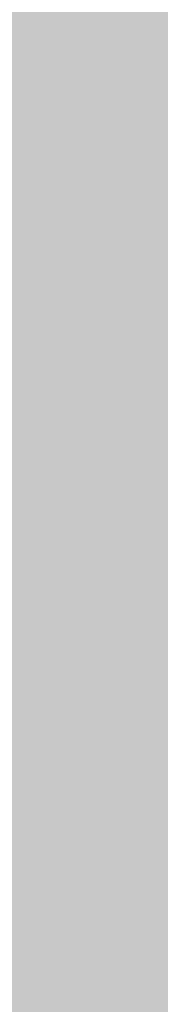
# Model space of a CAD drawing. Units: inches. Extents: x 2083 to 3317, y 1141 to 2115.
# Tile 179 of 256: x 3126.94671 to 3126.95594, y 1263.29018 to 1263.35483. Entities that reach past the tile are written whole.
import ezdxf

# ---------------------------------------------------------------- set-up
doc = ezdxf.new("R2010")
doc.units = ezdxf.units.IN
doc.layers.add('A-ANNO-DIMS', color=2, linetype='Continuous', lineweight=18)
doc.layers.add('A-WALL-PATT', color=251, linetype='Continuous', lineweight=13, true_color=0x636466)
doc.styles.get("Standard").update_dxf_attribs({"font": 'arial.ttf'})
doc.dimstyles.new('ISO-25', dxfattribs={"dimtxt": 12, "dimasz": 12, "dimexe": 1.25, "dimexo": 0.625, "dimtad": 1, "dimlunit": 3, "dimtxsty": 'Standard', "dimcen": 2.5, "dimadec": 0, "dimazin": 0, "dimtfac": 1, "dimtmove": 0, "dimatfit": 3, "dimfxl": 1, "dimarcsym": 0})

# ---------------------------------------------------------------- blocks, each defined once
blk = doc.blocks.new('*D26')
at = {"layer": 'A-ANNO-DIMS', "color": 0, "lineweight": -2, "transparency": 16777216}
for p, q in [((3088.985844, 1274.915092), (3088.985844, 1270.951963)), ((3111.240037, 1274.915092), (3111.240037, 1270.951963)), ((3076.985844, 1272.201963), (2840.262447, 1272.201963)), ((3111.240037, 1272.201963), (3088.985844, 1272.201963)), ((3123.240037, 1272.201963), (3135.240037, 1272.201963))]:
    blk.add_line(p, q, dxfattribs=at)
at = {"layer": 'A-ANNO-DIMS', "color": 0, "transparency": 16777216}
for points in [[(3076.985844, 1274.201963), (3076.985844, 1270.201963), (3088.985844, 1272.201963)], [(3123.240037, 1274.201963), (3123.240037, 1270.201963), (3111.240037, 1272.201963)]]:
    blk.add_solid(points, dxfattribs=at)
at = {"layer": 'Defpoints', "color": 0, "transparency": 16777216}
for p in [(3088.985844, 1275.540092), (3111.240037, 1275.540092), (3088.985844, 1272.201963)]:
    blk.add_point(p, dxfattribs=at)
at = {"layer": 'A-ANNO-DIMS', "color": 0, "transparency": 16777216, "insert": (2952.624146, 1279.031602), "char_height": 12, "attachment_point": 5}
blk.add_mtext('NIGHTSTAND 1\'-10 1/2" TYP.', dxfattribs=at)
blk = doc.blocks.new('*D27')
at = {"layer": 'A-ANNO-DIMS', "color": 0, "lineweight": -2, "transparency": 16777216}
for p, q in [((3114.578165, 1309.794285), (3114.578165, 1321.794285)), ((3111.865037, 1297.794285), (3115.828165, 1297.794285)), ((3114.578165, 1297.794285), (3114.578165, 1275.540092)), ((3111.865037, 1275.540092), (3115.828165, 1275.540092)), ((3114.578165, 1263.540092), (3114.578165, 1140.988591))]:
    blk.add_line(p, q, dxfattribs=at)
at = {"layer": 'A-ANNO-DIMS', "color": 0, "transparency": 16777216}
for points in [[(3112.578165, 1309.794285), (3116.578165, 1309.794285), (3114.578165, 1297.794285)], [(3112.578165, 1263.540092), (3116.578165, 1263.540092), (3114.578165, 1275.540092)]]:
    blk.add_solid(points, dxfattribs=at)
at = {"layer": 'Defpoints', "color": 0, "transparency": 16777216}
for p in [(3111.240037, 1297.794285), (3111.240037, 1275.540092), (3114.578165, 1275.540092)]:
    blk.add_point(p, dxfattribs=at)
at = {"layer": 'A-ANNO-DIMS', "color": 0, "transparency": 16777216, "insert": (3107.748527, 1196.264342), "char_height": 12, "attachment_point": 5, "rotation": 90}
blk.add_mtext('1\'-10 1/2" TYP.', dxfattribs=at)

msp = doc.modelspace()

# ---------------------------------------------------------------- hatches: boundary and pattern name
at = {"layer": 'A-WALL-PATT'}
h = msp.add_hatch(color=256, dxfattribs=at)
h.dxf.hatch_style = 1
h.paths.add_polyline_path([(3126.959783, 2020.76136), (2748.959783, 2020.76136), (2604.959783, 2020.76136), (2226.959783, 2020.76136), (2226.959783, 1702.76136), (2466.959783, 1702.76136), (2466.959783, 1582.76136), (2418.959783, 1582.76136), (2418.959783, 1477.76136), (2226.959783, 1477.76136), (2226.959783, 1263.26136), (2544.959783, 1263.26136), (2544.959783, 1411.76136), (2604.959783, 1411.76136), (2685.959783, 1411.76136), (2685.959783, 1420.76136), (2604.959783, 1420.76136), (2604.959783, 1573.76136), (2604.959783, 1702.76136), (2604.959783, 2011.76136), (2748.959783, 2011.76136), (2748.959783, 1702.76136), (2862.959783, 1702.76136), (2862.959783, 1621.76136), (2871.959783, 1621.76136), (2871.959783, 1702.76136), (2883.959783, 1702.76136), (2883.959783, 1706.939459, -0.026459), (2883.959783, 1711.76136), (2757.959783, 1711.76136), (2757.959783, 1807.76136), (2787.959783, 1807.76136), (2787.959783, 1812.26136), (2757.959783, 1812.26136), (2757.959783, 2011.76136), (2877.959783, 2011.76136), (2877.959783, 1812.26136), (2847.959783, 1812.26136), (2847.959783, 1807.76136), (2889.835742, 1807.76136), (2889.835742, 1812.26136), (2882.459783, 1812.26136), (2882.459783, 2011.76136), (3117.959783, 2011.76136), (3117.959783, 1812.26136), (2937.835742, 1812.26136), (2937.835742, 1807.76136), (2995.709783, 1807.76136), (2995.709783, 1796.117666), (3000.209783, 1796.117666), (3000.209783, 1807.76136), (3117.959783, 1807.76136), (3117.959783, 1711.76136), (3000.209783, 1711.76136), (3000.209783, 1760.117666), (2998.572705, 1760.117666, -0.020711), (2995.709783, 1760.117666), (2995.709783, 1711.76136), (2931.959783, 1711.76136), (2931.959783, 1702.76136), (3126.959783, 1702.76136)])
h.paths.add_polyline_path([(2471.459783, 2011.76136), (2471.459783, 1810.01136), (2462.716936, 1810.01136), (2462.716936, 1805.51136), (2505.959783, 1805.51136), (2505.959783, 1810.01136), (2475.959783, 1810.01136), (2475.959783, 2011.76136), (2595.959783, 2011.76136), (2595.959783, 1810.01136), (2565.959783, 1810.01136), (2565.959783, 1805.51136), (2595.959783, 1805.51136), (2595.959783, 1711.76136), (2235.959783, 1711.76136), (2235.959783, 1805.51136), (2353.709783, 1805.51136), (2353.709783, 1796.054162), (2358.209783, 1796.054162), (2358.209783, 1805.51136), (2414.716936, 1805.51136), (2414.716936, 1810.01136), (2235.959783, 1810.01136), (2235.959783, 2011.76136)], flags=16)
h.paths.add_polyline_path([(2270.204734, 1994.610008), (2270.204734, 1970.610008), (2246.204734, 1970.610008), (2246.204734, 1994.610008)], flags=0)
edge = h.paths.add_edge_path(flags=0)
edge.add_ellipse((2332.027391, 1899.798176), major_axis=(-3.042994, 3.042994), ratio=0.16825245, start_angle=-161.332166, end_angle=-156.307114, ccw=False)
edge.add_ellipse((2333.082037, 1898.74353), major_axis=(-1.054646, 1.054646), ratio=0.4535321, start_angle=-123.371019, end_angle=-94.159107)
edge = h.paths.add_edge_path(flags=0)
edge.add_ellipse((2332.027391, 1968.87629), major_axis=(3.042994, 3.042994), ratio=0.16825245, start_angle=18.667834, end_angle=23.692886)
edge.add_spline(control_points=[(2332.925596, 1970.691105), (2332.226768, 1970.3361), (2330.893709, 1969.658905), (2328.41308, 1970.932138), (2327.203934, 1967.748712), (2324.709596, 1969.955589), (2322.532822, 1967.012354), (2320.012846, 1971.295812), (2317.680308, 1968.157845), (2316.040526, 1967.102047), (2315.426904, 1966.809602)], knot_values=[0, 0, 0, 0, 2.267059, 4.324559, 6.685584, 8.878641, 11.121502, 14.300359, 17.755284, 19.732645, 19.732645, 19.732645, 19.732645], degree=3, periodic=0)
edge.add_ellipse((2332.027391, 1968.87629), major_axis=(3.042994, 3.042994), ratio=0.16825245, start_angle=18.667834, end_angle=23.692886, ccw=False)
edge.add_ellipse((2333.082037, 1969.930936), major_axis=(1.054646, 1.054646), ratio=0.4535321, start_angle=56.628981, end_angle=85.840893, ccw=False)
edge = h.paths.add_edge_path(flags=0)
edge.add_spline(control_points=[(2296.428287, 1967.987908), (2293.627804, 1965.336314), (2287.703624, 1959.727094), (2299.74386, 1949.995699), (2294.532591, 1935.668528), (2290.573228, 1920.603512), (2293.394124, 1909.973691), (2296.185407, 1904.966543)], knot_values=[0.099185, 0.099185, 0.099185, 0.099185, 0.345301, 0.619822, 0.982653, 1.386093, 1.810555, 1.810555, 1.810555, 1.810555], degree=3, periodic=0)
edge.add_spline(control_points=[(2296.185407, 1904.966543), (2297.383582, 1902.6193), (2298.000969, 1901.949312), (2298.55297, 1901.468155)], knot_values=[0.006246, 0.006246, 0.006246, 0.006246, 0.055476, 0.055476, 0.055476, 0.055476], degree=3, periodic=0)
edge.add_spline(control_points=[(2298.55297, 1901.468155), (2297.258612, 1900.923224), (2295.225294, 1900.232126), (2293.060229, 1900.614205), (2292.101423, 1900.788415), (2292.089578, 1900.790568)], knot_values=[0.312835, 0.312835, 0.312835, 0.312835, 0.40178, 0.474987, 0.475903, 0.475903, 0.475903, 0.475903], degree=3, periodic=0)
edge.add_arc((2292.793646, 1904.664109), 3.937008, 215.420897, 259.698179, ccw=False)
edge.add_spline(control_points=[(2289.585314, 1902.382304), (2289.476652, 1902.535087), (2289.36848, 1902.688035), (2289.260865, 1902.84117)], knot_values=[0.102872, 0.102872, 0.102872, 0.102872, 0.116896, 0.116896, 0.116896, 0.116896], degree=3, periodic=0)
edge.add_spline(control_points=[(2289.260865, 1902.84117), (2288.686604, 1902.550192), (2287.640048, 1902.019902), (2285.881337, 1901.873954), (2283.852972, 1901.504352), (2281.719987, 1899.710538), (2278.466991, 1899.492942), (2276.157136, 1901.883202), (2272.258953, 1899.804071), (2267.777605, 1901.843183), (2262.243882, 1900.184033), (2257.414927, 1901.782061), (2254.318374, 1900.72612), (2253.178285, 1900.337343)], knot_values=[0, 0, 0, 0, 1.907977, 3.477176, 5.261074, 7.972851, 11.680248, 13.717921, 16.939592, 22.789562, 27.502503, 33.595215, 37.145618, 37.145618, 37.145618, 37.145618], degree=3, periodic=0)
edge.add_line((2253.178285, 1900.337343), (2250.24424, 1902.84117))
edge.add_line((2250.24424, 1902.84117), (2250.24424, 1965.833296))
edge.add_line((2250.24424, 1965.833296), (2253.178285, 1968.337123))
edge.add_spline(control_points=[(2253.178285, 1968.337123), (2254.318374, 1967.948346), (2257.414927, 1966.892405), (2262.243882, 1968.490433), (2267.777605, 1966.831283), (2271.52673, 1968.537217), (2273.875914, 1967.828289), (2274.206701, 1967.727642)], knot_values=[0, 0, 0, 0, 0.09018, 0.244935, 0.364644, 0.513233, 0.537855, 0.537855, 0.537855, 0.537855], degree=3, periodic=0)
edge.add_arc((2274.352887, 1963.793349), 3.937008, 72.051134, 92.127949, ccw=False)
edge.add_arc((2281.296933, 1985.230003), 18.596298, 252.0511336, 288.5657217)
edge.add_arc((2292.316717, 1956.02888), 12.646081, 71.0267879, 113.7782184, ccw=False)
edge = h.paths.add_edge_path(flags=0)
edge.add_spline(control_points=[(2274.899415, 1951.856195), (2275.066156, 1951.616592), (2275.232687, 1951.376588), (2275.397987, 1951.135855)], knot_values=[1.409916, 1.409916, 1.409916, 1.409916, 1.43159, 1.43159, 1.43159, 1.43159], degree=3, periodic=0)
edge.add_spline(control_points=[(2275.397987, 1951.135855), (2275.792106, 1950.561885), (2276.179231, 1949.983774), (2276.545546, 1949.397103)], knot_values=[1.358238, 1.358238, 1.358238, 1.358238, 1.409916, 1.409916, 1.409916, 1.409916], degree=3, periodic=0)
edge.add_line((2276.545546, 1949.397103), (2277.437289, 1947.862185))
edge.add_spline(control_points=[(2277.437289, 1947.862185), (2276.303834, 1945.673115), (2274.639698, 1942.426882), (2274.631615, 1938.0939), (2272.799124, 1930.85155), (2274.356426, 1943.897046), (2275.947681, 1947.923356), (2276.545546, 1949.397103)], knot_values=[0.005632, 0.005632, 0.005632, 0.005632, 0.186014, 0.266002, 0.357087, 0.59639, 0.739732, 0.739732, 0.739732, 0.739732], degree=3, periodic=0)
edge.add_spline(control_points=[(2276.545546, 1949.397103), (2276.179231, 1949.983774), (2275.792106, 1950.561885), (2275.397987, 1951.135855)], knot_values=[1.358238, 1.358238, 1.358238, 1.358238, 1.409916, 1.409916, 1.409916, 1.409916], degree=3, periodic=0)
edge.add_spline(control_points=[(2275.397987, 1951.135855), (2274.9425, 1950.080452), (2274.20776, 1948.025272), (2273.934602, 1944.851477), (2272.468534, 1937.627489), (2273.466216, 1945.696466), (2274.700615, 1951.059472), (2274.899415, 1951.856195)], knot_values=[0.104364, 0.104364, 0.104364, 0.104364, 0.189636, 0.269624, 0.36071, 0.600013, 0.644622, 0.644622, 0.644622, 0.644622], degree=3, periodic=0)
h.paths.add_polyline_path([(2269.167514, 1963.127573, -0.357527), (2268.170633, 1960.97637, -0.092561), (2268.170633, 1939.436325, -0.357527), (2269.167514, 1937.285122, -0.357527), (2267.01631, 1938.282002, -0.164785), (2254.685581, 1938.282002, -0.357527), (2252.534378, 1937.285122, -0.357527), (2253.531259, 1939.436325, -0.092561), (2253.531259, 1960.97637, -0.357527), (2252.534378, 1963.127573, -0.357527), (2254.685581, 1962.130692, -0.164785), (2267.01631, 1962.130692, -0.357527)], flags=0)
h.paths.add_polyline_path([(2248.874068, 1967.8018), (2248.874068, 1957.02771), (2249.457783, 1957.02771), (2249.457783, 1911.646756), (2248.874068, 1911.646756), (2248.874068, 1900.872666), (2246.511863, 1900.872666, 0.197327), (2244.149658, 1902.456873), (2244.149658, 1966.217592, 0.197327), (2246.511863, 1967.8018)], flags=0)
h.paths.add_polyline_path([(2269.167514, 1931.389344, -0.357527), (2268.170633, 1929.238141, -0.092561), (2268.170633, 1907.698096, -0.357527), (2269.167514, 1905.546893, -0.357527), (2267.01631, 1906.543774, -0.164785), (2254.685581, 1906.543774, -0.357527), (2252.534378, 1905.546893, -0.357527), (2253.531259, 1907.698096, -0.092561), (2253.531259, 1929.238141, -0.357527), (2252.534378, 1931.389344, -0.357527), (2254.685581, 1930.392463, -0.164785), (2267.01631, 1930.392463, -0.357527)], flags=0)
edge = h.paths.add_edge_path(flags=0)
edge.add_spline(control_points=[(2276.196858, 1906.723702), (2276.168144, 1909.028928), (2276.114049, 1913.371852), (2270.598417, 1924.924978), (2273.905175, 1919.012779), (2275.921711, 1916.262063), (2275.47457, 1912.402149), (2277.257874, 1910.380621), (2276.696044, 1908.225036), (2276.646218, 1906.813023), (2276.617825, 1906.008407)], knot_values=[0, 0, 0, 0, 8.61026, 16.221274, 18.843057, 23.804898, 27.440828, 29.356102, 31.203478, 33.650687, 33.650687, 33.650687, 33.650687], degree=3, periodic=0)
edge.add_spline(control_points=[(2276.617825, 1906.008407), (2276.623313, 1905.624144), (2276.497738, 1904.628661), (2275.441779, 1903.854725), (2274.937314, 1903.08045), (2274.85908, 1902.84117)], knot_values=[0.156488, 0.156488, 0.156488, 0.156488, 0.184398, 0.231376, 0.250598, 0.250598, 0.250598, 0.250598], degree=3, periodic=0)
edge.add_line((2274.85908, 1902.84117), (2276.50598, 1902.84117))
edge.add_spline(control_points=[(2276.50598, 1902.84117), (2276.788308, 1903.08494), (2277.665071, 1904.125196), (2278.249538, 1904.340738), (2277.653872, 1908.527387), (2278.15567, 1906.227808), (2278.100464, 1905.285948), (2278.846675, 1904.069005), (2277.856785, 1903.414948), (2277.874191, 1902.99105), (2277.903562, 1902.84117)], knot_values=[0.059574, 0.059574, 0.059574, 0.059574, 0.080753, 0.103741, 0.16972, 0.176036, 0.207137, 0.240474, 0.262341, 0.27366, 0.27366, 0.27366, 0.27366], degree=3, periodic=0)
edge.add_line((2277.903562, 1902.84117), (2280.029825, 1902.84117))
edge.add_spline(control_points=[(2280.029825, 1902.84117), (2279.888221, 1903.088398), (2279.499257, 1903.981551), (2280.152284, 1905.939349), (2278.103615, 1909.657757), (2279.762395, 1907.185285), (2280.3279, 1904.874861), (2280.485109, 1903.48959), (2281.463269, 1903.249432), (2281.758343, 1902.936497), (2281.834036, 1902.84117)], knot_values=[0.013856, 0.013856, 0.013856, 0.013856, 0.034874, 0.088867, 0.107879, 0.126738, 0.158714, 0.193757, 0.217487, 0.226722, 0.226722, 0.226722, 0.226722], degree=3, periodic=0)
edge.add_spline(control_points=[(2281.834036, 1902.84117), (2281.787535, 1902.826703), (2281.647022, 1902.782988), (2281.395527, 1902.85949), (2281.088077, 1902.985242), (2280.720683, 1903.060902), (2280.333451, 1903.025726), (2280.124767, 1902.898879), (2280.029825, 1902.84117)], knot_values=[0, 0, 0, 0, 0.14413, 0.435517, 0.749276, 1.153046, 1.548371, 1.878348, 1.878348, 1.878348, 1.878348], degree=3, periodic=0)
edge.add_line((2280.029825, 1902.84117), (2277.903562, 1902.84117))
edge.add_spline(control_points=[(2277.903562, 1902.84117), (2277.892855, 1902.795855), (2277.865396, 1902.679637), (2277.607479, 1902.687483), (2277.27405, 1902.8007), (2276.837921, 1902.619775), (2276.583807, 1902.789261), (2276.50598, 1902.84117)], knot_values=[0, 0, 0, 0, 0.127189, 0.326199, 0.628009, 1.24357, 1.515331, 1.515331, 1.515331, 1.515331], degree=3, periodic=0)
edge.add_line((2276.50598, 1902.84117), (2274.85908, 1902.84117))
edge.add_spline(control_points=[(2274.85908, 1902.84117), (2274.814437, 1902.898587), (2274.72513, 1903.013446), (2274.493477, 1903.118968), (2274.244285, 1902.960539), (2273.937121, 1903.184942), (2273.614039, 1902.983143), (2273.408316, 1902.883045), (2273.322254, 1902.84117)], knot_values=[0, 0, 0, 0, 0.21843, 0.436957, 0.687977, 0.990379, 1.398396, 1.69185, 1.69185, 1.69185, 1.69185], degree=3, periodic=0)
edge.add_spline(control_points=[(2273.322254, 1902.84117), (2273.61674, 1903.445692), (2274.273998, 1904.538253), (2276.027239, 1904.573702), (2276.206963, 1906.583637), (2276.196858, 1906.723702)], knot_values=[0.012227, 0.012227, 0.012227, 0.012227, 0.059472, 0.106218, 0.134458, 0.134458, 0.134458, 0.134458], degree=3, periodic=0)
h.paths.add_polyline_path([(2270.776054, 1897.789828), (2270.776054, 1873.789828), (2246.776054, 1873.789828), (2246.776054, 1897.789828)], flags=0)
h.paths.add_polyline_path([(2353.709783, 1760.005059), (2353.709783, 1760.054162), (2358.209783, 1760.054162, -0.033729)], flags=0)
h.paths.add_polyline_path([(2321.819119, 1737.529186), (2341.995327, 1737.529186, -0.414214), (2343.203273, 1736.321241), (2343.203273, 1721.020596, -0.414214), (2341.995327, 1719.812651), (2321.819119, 1719.812651, -0.414214), (2320.611173, 1721.020596), (2320.611173, 1736.321241, -0.414214)], flags=0)
h.paths.add_polyline_path([(2324.23501, 1736.321241), (2339.579436, 1736.321241, -0.414214), (2341.995327, 1733.905349), (2341.995327, 1725.44973, -0.414214), (2339.579436, 1723.033839), (2333.680588, 1723.033839), (2333.845317, 1722.045467, -0.870646), (2335.425399, 1721.825893, -0.767327), (2333.922694, 1721.423245), (2331.291024, 1721.423245, -0.767327), (2329.788319, 1721.825893, -0.870646), (2331.368401, 1722.045467), (2331.53313, 1723.033839), (2324.23501, 1723.033839, -0.414214), (2321.819119, 1725.44973), (2321.819119, 1733.905349, -0.414214)], flags=0)
h.paths.add_polyline_path([(2570.483789, 1928.615444), (2589.683789, 1928.615444), (2590.168829, 1928.615444), (2590.168829, 1904.993397), (2570.483789, 1904.993397)], flags=0)
h.paths.add_polyline_path([(2574.447324, 1927.263822, -1), (2572.828836, 1927.263822, -1)], flags=0)
h.paths.add_polyline_path([(2573.089867, 1926.940877), (2573.925032, 1927.776042), (2574.147743, 1927.553332), (2573.312577, 1926.718166)], flags=0)
h.paths.add_polyline_path([(2578.779065, 1919.729618, -1), (2571.591663, 1919.729618, -1)], flags=0)
h.paths.add_polyline_path([(2578.385364, 1919.729618, -1), (2571.985364, 1919.729618, -1)], flags=0)
h.paths.add_polyline_path([(2331.595764, 1729.476216, -1), (2333.617954, 1729.476216, -1)], flags=0)
h.paths.add_polyline_path([(2578.034228, 1927.263822, -1), (2576.41574, 1927.263822, -1)], flags=0)
h.paths.add_polyline_path([(2576.688851, 1927.531089), (2576.911562, 1927.753799), (2577.746728, 1926.918634), (2577.524017, 1926.695923)], flags=0)
h.paths.add_polyline_path([(2578.139065, 1909.859539, -1), (2572.231663, 1909.859539, -1)], flags=0)
h.paths.add_polyline_path([(2577.745364, 1909.859539, -1), (2572.625364, 1909.859539, -1)], flags=0)
h.paths.add_polyline_path([(2583.797718, 1927.263822, -1), (2582.179229, 1927.263822, -1)], flags=0)
h.paths.add_polyline_path([(2582.718649, 1927.753799), (2583.553814, 1926.918634), (2583.331103, 1926.695923), (2582.495938, 1927.531089)], flags=0)
h.paths.add_polyline_path([(2582.495938, 1927.531089), (2582.718649, 1927.753799), (2583.553814, 1926.918634), (2583.331103, 1926.695923)], flags=0)
h.paths.add_polyline_path([(2587.739065, 1920.529618, -1), (2581.831663, 1920.529618, -1)], flags=0)
h.paths.add_polyline_path([(2587.345364, 1920.529618, -1), (2582.225364, 1920.529618, -1)], flags=0)
h.paths.add_polyline_path([(2587.384622, 1927.263822, -1), (2585.766133, 1927.263822, -1)], flags=0)
h.paths.add_polyline_path([(2586.081993, 1926.980247), (2586.917158, 1927.815412), (2587.139869, 1927.592702), (2586.304703, 1926.757536)], flags=0)
h.paths.add_polyline_path([(2588.379065, 1910.659539, -1), (2581.191663, 1910.659539, -1)], flags=0)
h.paths.add_polyline_path([(2587.985364, 1910.659539, -1), (2581.585364, 1910.659539, -1)], flags=0)
h.paths.add_polyline_path([(2417.167729, 1729.477895), (2437.343937, 1729.477895, -0.414214), (2438.551883, 1728.26995), (2438.551883, 1712.969306, -0.414214), (2437.343937, 1711.76136), (2417.167729, 1711.76136, -0.414214), (2415.959783, 1712.969306), (2415.959783, 1728.26995, -0.414214)], flags=0)
h.paths.add_polyline_path([(2419.58362, 1728.26995), (2434.928046, 1728.26995, -0.414214), (2437.343937, 1725.854059), (2437.343937, 1717.39844, -0.414214), (2434.928046, 1714.982548), (2429.029199, 1714.982548), (2429.193927, 1713.994176, -0.870646), (2430.774009, 1713.774603, -0.767327), (2429.271304, 1713.371954), (2426.639634, 1713.371954, -0.767327), (2425.136929, 1713.774603, -0.870646), (2426.717011, 1713.994176), (2426.88174, 1714.982548), (2419.58362, 1714.982548, -0.414214), (2417.167729, 1717.39844), (2417.167729, 1725.854059, -0.414214)], flags=0)
h.paths.add_polyline_path([(2419.58362, 1728.26995), (2434.928046, 1728.26995, -0.414214), (2437.343937, 1725.854059), (2437.343937, 1717.39844, -0.414214), (2434.928046, 1714.982548), (2429.029199, 1714.982548), (2428.358118, 1719.009034), (2427.552821, 1719.009034), (2426.88174, 1714.982548), (2419.58362, 1714.982548, -0.414214), (2417.167729, 1717.39844), (2417.167729, 1725.854059, -0.414214)], flags=0)
h.paths.add_polyline_path([(2426.944374, 1721.424925, -1), (2428.966564, 1721.424925, -1)], flags=0)
h.paths.add_polyline_path([(2475.959783, 1702.76136), (2595.959783, 1702.76136), (2595.959783, 1582.76136), (2475.959783, 1582.76136)], flags=16)
h.paths.add_polyline_path([(2427.959783, 1573.76136), (2595.959783, 1573.76136), (2595.959783, 1468.76136), (2595.959783, 1420.76136), (2384.459783, 1420.76136), (2384.459783, 1468.76136), (2427.959783, 1468.76136)], flags=16)
h.paths.add_polyline_path([(2379.959783, 1468.76136), (2379.959783, 1420.76136), (2235.959783, 1420.76136), (2235.959783, 1468.76136)], flags=16)
h.paths.add_polyline_path([(2317.815996, 1466.695767), (2337.992205, 1466.695767, -0.414214), (2339.20015, 1465.487821), (2339.20015, 1450.187177, -0.414214), (2337.992205, 1448.979232), (2317.815996, 1448.979232, -0.414214), (2316.608051, 1450.187177), (2316.608051, 1465.487821, -0.414214)], flags=0)
h.paths.add_polyline_path([(2320.231887, 1465.487821), (2335.576313, 1465.487821, -0.414214), (2337.992205, 1463.07193), (2337.992205, 1454.616311, -0.414214), (2335.576313, 1452.20042), (2329.677466, 1452.20042), (2329.842195, 1451.212047, -0.870646), (2331.422276, 1450.992474, -0.767327), (2329.919571, 1450.589826), (2327.287902, 1450.589826, -0.767327), (2325.785197, 1450.992474, -0.870646), (2327.365278, 1451.212047), (2327.530007, 1452.20042), (2320.231887, 1452.20042, -0.414214), (2317.815996, 1454.616311), (2317.815996, 1463.07193, -0.414214)], flags=0)
h.paths.add_polyline_path([(2320.231887, 1465.487821), (2335.576313, 1465.487821, -0.414214), (2337.992205, 1463.07193), (2337.992205, 1454.616311, -0.414214), (2335.576313, 1452.20042), (2329.677466, 1452.20042), (2329.006385, 1456.226905), (2328.201088, 1456.226905), (2327.530007, 1452.20042), (2320.231887, 1452.20042, -0.414214), (2317.815996, 1454.616311), (2317.815996, 1463.07193, -0.414214)], flags=0)
h.paths.add_polyline_path([(2327.592641, 1458.642796, -1), (2329.614832, 1458.642796, -1)], flags=0)
h.paths.add_polyline_path([(2244.411744, 1433.340453), (2241.920945, 1433.340453, -0.414214), (2240.017856, 1435.243542), (2240.017856, 1440.952808, -0.414211), (2241.920925, 1442.855897), (2244.411744, 1442.855897, -1.976472)], flags=0)
h.paths.add_polyline_path([(2245.356888, 1434.397536, -0.414214), (2245.356888, 1441.798814, -2.144098)], flags=0)
h.paths.add_polyline_path([(2535.959783, 1416.26136), (2535.959783, 1272.26136), (2235.959783, 1272.26136), (2235.959783, 1416.26136)], flags=16)
h.paths.add_polyline_path([(2260.119561, 1384.292841), (2260.119561, 1362.038649), (2237.865369, 1362.038649), (2237.865369, 1384.292841)], flags=0)
edge = h.paths.add_edge_path(flags=0)
edge.add_line((2318.251847, 1362.093298), (2318.145797, 1362.000973))
edge.add_ellipse((2317.445116, 1360.431044), major_axis=(2.82164, 2.82164), ratio=0.16825245, start_angle=18.667834, end_angle=20.948127, ccw=False)
edge.add_ellipse((2318.423045, 1361.408974), major_axis=(0.977929, 0.977929), ratio=0.4535321, start_angle=56.628981, end_angle=70.226201, ccw=False)
edge = h.paths.add_edge_path(flags=0)
edge.add_line((2319.10737, 1295.571078), (2319.015044, 1295.677128))
edge.add_ellipse((2317.445116, 1296.377809), major_axis=(-2.82164, 2.82164), ratio=0.16825245, start_angle=-161.332166, end_angle=-159.051873, ccw=False)
edge.add_ellipse((2318.423045, 1295.39988), major_axis=(-0.977929, 0.977929), ratio=0.4535321, start_angle=-123.371019, end_angle=-109.773799)
edge = h.paths.add_edge_path(flags=0)
edge.add_spline(control_points=[(2284.210349, 1301.170219), (2284.580688, 1300.444719), (2284.891189, 1299.892024), (2285.159553, 1299.461018)], knot_values=[0.039066, 0.039066, 0.039066, 0.039066, 0.055476, 0.055476, 0.055476, 0.055476], degree=3, periodic=0)
edge.add_line((2285.159553, 1299.461018), (2284.210349, 1301.170219))
edge = h.paths.add_edge_path(flags=0)
edge.add_line((2280.412458, 1297.298013), (2283.369991, 1297.036122))
edge.add_line((2283.369991, 1297.036122), (2286.40569, 1297.92631))
edge.add_spline(control_points=[(2286.40569, 1297.92631), (2285.305487, 1297.463119), (2284.344777, 1297.129151), (2283.369991, 1297.036122)], knot_values=[0.394369, 0.394369, 0.394369, 0.394369, 0.475903, 0.475903, 0.475903, 0.475903], degree=3, periodic=0)
edge.add_spline(control_points=[(2283.369991, 1297.036122), (2283.28139, 1297.027666), (2282.316289, 1296.957336), (2281.312502, 1297.134479), (2280.423441, 1297.296016), (2280.412458, 1297.298013)], knot_values=[0.312835, 0.312835, 0.312835, 0.312835, 0.320246, 0.393453, 0.394369, 0.394369, 0.394369, 0.394369], degree=3, periodic=0)
edge = h.paths.add_edge_path(flags=0)
edge.add_line((2284.435561, 1359.607285), (2280.446291, 1355.328047))
edge.add_line((2280.446291, 1355.328047), (2279.579987, 1351.017754))
edge.add_line((2279.579987, 1351.017754), (2282.412974, 1346.580433))
edge.add_spline(control_points=[(2282.412974, 1346.580433), (2283.153331, 1345.589236), (2284.252896, 1344.028897), (2284.801037, 1342.387167), (2284.935162, 1341.805544)], knot_values=[1.240098, 1.240098, 1.240098, 1.240098, 1.332892, 1.382712, 1.382712, 1.382712, 1.382712], degree=3, periodic=0)
edge.add_spline(control_points=[(2284.935162, 1341.805544), (2285.319108, 1340.1406), (2285.233029, 1338.409204), (2284.909938, 1336.654122)], knot_values=[1.097484, 1.097484, 1.097484, 1.097484, 1.240098, 1.240098, 1.240098, 1.240098], degree=3, periodic=0)
edge.add_spline(control_points=[(2284.909938, 1336.654122), (2284.586848, 1334.89904), (2284.026745, 1333.120272), (2283.462644, 1331.360585)], knot_values=[0.95487, 0.95487, 0.95487, 0.95487, 1.097484, 1.097484, 1.097484, 1.097484], degree=3, periodic=0)
edge.add_line((2283.462644, 1331.360585), (2281.890376, 1326.153357))
edge.add_line((2281.890376, 1326.153357), (2280.756259, 1321.056089))
edge.add_line((2280.756259, 1321.056089), (2280.299205, 1316.001977))
edge.add_line((2280.299205, 1316.001977), (2280.715933, 1310.950068))
edge.add_line((2280.715933, 1310.950068), (2282.028094, 1305.972137))
edge.add_line((2282.028094, 1305.972137), (2284.210349, 1301.170219))
edge.add_spline(control_points=[(2284.210349, 1301.170219), (2283.340731, 1302.730185), (2282.611904, 1304.336493), (2282.028094, 1305.972137)], knot_values=[0.099185, 0.099185, 0.099185, 0.099185, 0.241799, 0.241799, 0.241799, 0.241799], degree=3, periodic=0)
edge.add_spline(control_points=[(2282.028094, 1305.972137), (2281.444283, 1307.60778), (2281.005489, 1309.272759), (2280.715933, 1310.950068)], knot_values=[0.241799, 0.241799, 0.241799, 0.241799, 0.384413, 0.384413, 0.384413, 0.384413], degree=3, periodic=0)
edge.add_spline(control_points=[(2280.715933, 1310.950068), (2280.433241, 1312.587613), (2280.289386, 1314.276959), (2280.298894, 1315.962032), (2280.299205, 1316.001977)], knot_values=[0.384413, 0.384413, 0.384413, 0.384413, 0.523647, 0.527028, 0.527028, 0.527028, 0.527028], degree=3, periodic=0)
edge.add_spline(control_points=[(2280.299205, 1316.001977), (2280.312326, 1317.686955), (2280.477871, 1319.367926), (2280.756259, 1321.056089)], knot_values=[0.527028, 0.527028, 0.527028, 0.527028, 0.669642, 0.669642, 0.669642, 0.669642], degree=3, periodic=0)
edge.add_spline(control_points=[(2280.756259, 1321.056089), (2281.034648, 1322.744252), (2281.42588, 1324.439608), (2281.890376, 1326.153357)], knot_values=[0.669642, 0.669642, 0.669642, 0.669642, 0.812256, 0.812256, 0.812256, 0.812256], degree=3, periodic=0)
edge.add_spline(control_points=[(2281.890376, 1326.153357), (2282.264383, 1327.533251), (2282.78787, 1329.26181), (2283.352751, 1331.01778), (2283.462644, 1331.360585)], knot_values=[0.812256, 0.812256, 0.812256, 0.812256, 0.927087, 0.95487, 0.95487, 0.95487, 0.95487], degree=3, periodic=0)
edge.add_line((2283.462644, 1331.360585), (2284.909938, 1336.654122))
edge.add_line((2284.909938, 1336.654122), (2284.935162, 1341.805544))
edge.add_line((2284.935162, 1341.805544), (2282.412974, 1346.580433))
edge.add_spline(control_points=[(2282.412974, 1346.580433), (2281.275127, 1348.103792), (2280.078447, 1349.570318), (2279.579987, 1351.017754)], knot_values=[1.382712, 1.382712, 1.382712, 1.382712, 1.525326, 1.525326, 1.525326, 1.525326], degree=3, periodic=0)
edge.add_spline(control_points=[(2279.579987, 1351.017754), (2279.443282, 1351.414721), (2279.136312, 1352.856922), (2279.73519, 1354.290385), (2280.446291, 1355.328047)], knot_values=[1.525326, 1.525326, 1.525326, 1.525326, 1.564439, 1.667941, 1.667941, 1.667941, 1.667941], degree=3, periodic=0)
edge.add_spline(control_points=[(2280.446291, 1355.328047), (2281.426113, 1356.757835), (2282.930837, 1358.18256), (2284.435561, 1359.607285)], knot_values=[1.667941, 1.667941, 1.667941, 1.667941, 1.810555, 1.810555, 1.810555, 1.810555], degree=3, periodic=0)
edge.add_arc((2280.623075, 1348.518181), 11.72618, 71.0267879, 113.7782184)
edge.add_arc((2270.404892, 1375.595156), 17.243567, 252.0511336, 288.5657217, ccw=False)
edge.add_arc((2263.965969, 1355.717847), 3.650622, 72.051134, 92.127949)
edge.add_arc((2263.965969, 1355.717847), 3.650622, 92.127949, 177.98513)
edge.add_spline(control_points=[(2260.317604, 1355.846199), (2260.260417, 1354.220668), (2260.551278, 1350.186547), (2262.999344, 1346.766251), (2264.472741, 1344.649024)], knot_values=[1.43159, 1.43159, 1.43159, 1.43159, 1.564144, 1.770695, 1.770695, 1.770695, 1.770695], degree=3, periodic=0)
edge.add_line((2264.472741, 1344.649024), (2264.93559, 1343.98253))
edge.add_spline(control_points=[(2263.801044, 1340.248105), (2263.843238, 1340.514088), (2264.067244, 1341.756465), (2264.512693, 1343.002453), (2264.935047, 1343.981083)], knot_values=[0.53657, 0.53657, 0.53657, 0.53657, 0.559349, 0.644622, 0.644622, 0.644622, 0.644622], degree=3, periodic=0)
edge.add_spline(control_points=[(2264.935047, 1343.981083), (2265.117771, 1343.714975), (2265.298875, 1343.447906), (2265.476756, 1343.179365)], knot_values=[1.384077, 1.384077, 1.384077, 1.384077, 1.409916, 1.409916, 1.409916, 1.409916], degree=3, periodic=0)
edge.add_spline(control_points=[(2265.476756, 1343.179365), (2265.654637, 1342.910823), (2265.829296, 1342.64081), (2265.99913, 1342.368812)], knot_values=[1.358238, 1.358238, 1.358238, 1.358238, 1.384077, 1.384077, 1.384077, 1.384077], degree=3, periodic=0)
edge.add_line((2265.99913, 1342.368812), (2266.826006, 1340.945547))
edge.add_spline(control_points=[(2266.826006, 1340.945547), (2268.894401, 1337.089691), (2271.398173, 1325.843001), (2270.516164, 1310.568557), (2275.919376, 1301.860609), (2277.789511, 1299.19945)], knot_values=[0.116896, 0.116896, 0.116896, 0.116896, 0.472987, 1.050969, 1.313793, 1.313793, 1.313793, 1.313793], degree=3, periodic=0)
edge.add_spline(control_points=[(2277.789511, 1299.19945), (2277.839405, 1299.128452), (2277.889428, 1299.057498), (2277.939572, 1298.986584)], knot_values=[0.109884, 0.109884, 0.109884, 0.109884, 0.116896, 0.116896, 0.116896, 0.116896], degree=3, periodic=0)
edge.add_line((2277.939572, 1298.986584), (2277.788849, 1299.199114))
edge.add_spline(control_points=[(2277.788849, 1299.199114), (2277.256582, 1298.929414), (2276.28635, 1298.437902), (2275.039352, 1298.334419), (2274.38333, 1298.238895), (2274.215254, 1298.209338)], knot_values=[33.12187, 33.12187, 33.12187, 33.12187, 35.029056, 36.598255, 37.144827, 37.144827, 37.144827, 37.144827], degree=3, periodic=0)
edge.add_line((2274.215254, 1298.209338), (2273.073147, 1297.892961))
edge.add_spline(control_points=[(2273.073147, 1297.892961), (2272.322936, 1297.579784), (2271.039151, 1296.510508), (2269.248395, 1296.226062), (2268.4231, 1296.374654)], knot_values=[26.532584, 26.532584, 26.532584, 26.532584, 29.198919, 31.839101, 31.839101, 31.839101, 31.839101], degree=3, periodic=0)
edge.add_line((2268.4231, 1296.374654), (2263.878501, 1297.457534))
edge.add_spline(control_points=[(2263.878501, 1297.457534), (2263.556077, 1297.359435), (2261.860306, 1296.838694), (2260.23878, 1297.282407), (2258.933454, 1297.516461)], knot_values=[15.919551, 15.919551, 15.919551, 15.919551, 16.939592, 21.226067, 21.226067, 21.226067, 21.226067], degree=3, periodic=0)
edge.add_line((2258.933454, 1297.516461), (2254.055233, 1297.32901))
edge.add_spline(control_points=[(2254.055233, 1297.32901), (2253.755525, 1297.295815), (2252.113683, 1297.165174), (2250.461869, 1297.544221), (2249.129686, 1297.667882)], knot_values=[5.306517, 5.306517, 5.306517, 5.306517, 6.276435, 10.613034, 10.613034, 10.613034, 10.613034], degree=3, periodic=0)
edge.add_line((2249.129686, 1297.667882), (2244.33165, 1296.877756))
edge.add_line((2244.33165, 1296.877756), (2241.611033, 1299.19945))
edge.add_line((2241.611033, 1299.19945), (2241.611033, 1357.609404))
edge.add_line((2241.611033, 1357.609404), (2244.33165, 1359.931097))
edge.add_line((2244.33165, 1359.931097), (2252.728823, 1359.542692))
edge.add_spline(control_points=[(2252.728823, 1359.542692), (2252.870939, 1359.54644), (2253.30574, 1359.548172), (2253.739845, 1359.514274), (2254.031742, 1359.482426)], knot_values=[0.233291, 0.233291, 0.233291, 0.233291, 0.244935, 0.268927, 0.268927, 0.268927, 0.268927], degree=3, periodic=0)
edge.add_line((2254.031742, 1359.482426), (2259.58719, 1359.41639))
edge.add_spline(control_points=[(2259.58719, 1359.41639), (2260.677068, 1359.628503), (2262.073197, 1359.897003), (2263.523692, 1359.459278), (2263.830417, 1359.365952)], knot_values=[0.422516, 0.422516, 0.422516, 0.422516, 0.513233, 0.537855, 0.537855, 0.537855, 0.537855], degree=3, periodic=0)
edge.add_arc((2263.965969, 1355.717847), 3.650622, 72.051134, 92.127949, ccw=False)
edge.add_arc((2270.404892, 1375.595156), 17.243567, 252.0511336, 288.5657217)
edge.add_arc((2280.623075, 1348.518181), 11.72618, 71.0267879, 113.7782184, ccw=False)
h.paths.add_polyline_path([(2240.34053, 1359.434715), (2240.34053, 1349.444353), (2240.881785, 1349.444353), (2240.881785, 1307.3645), (2240.34053, 1307.3645), (2240.34053, 1297.374138), (2238.150157, 1297.374138, 0.197327), (2235.959783, 1298.843108), (2235.959783, 1357.965746, 0.197327), (2238.150157, 1359.434715)], flags=0)
h.paths.add_polyline_path([(2259.15779, 1355.1005, -0.357527), (2258.233425, 1353.10578, -0.092561), (2258.233425, 1333.132601, -0.357527), (2259.15779, 1331.13788, -0.357527), (2257.16307, 1332.062246, -0.164785), (2245.729302, 1332.062246, -0.357527), (2243.734582, 1331.13788, -0.357527), (2244.658947, 1333.132601, -0.092561), (2244.658947, 1353.10578, -0.357527), (2243.734582, 1355.1005, -0.357527), (2245.729302, 1354.176135, -0.164785), (2257.16307, 1354.176135, -0.357527)], flags=0)
edge = h.paths.add_edge_path(flags=0)
edge.add_line((2265.99913, 1342.368812), (2266.826006, 1340.945547))
edge.add_line((2266.826006, 1340.945547), (2265.307557, 1337.814066))
edge.add_line((2265.307557, 1337.814066), (2264.358232, 1334.652939))
edge.add_line((2264.358232, 1334.652939), (2264.262012, 1333.799705))
edge.add_spline(control_points=[(2264.262012, 1333.799705), (2264.208357, 1333.187055), (2264.16206, 1332.365525), (2264.007144, 1331.413933), (2263.969049, 1331.201834)], knot_values=[0.464444, 0.464444, 0.464444, 0.464444, 0.516691, 0.531608, 0.531608, 0.531608, 0.531608], degree=3, periodic=0)
edge.add_spline(control_points=[(2263.969049, 1331.201834), (2263.774535, 1330.118873), (2263.42437, 1328.790839), (2263.25742, 1328.530652), (2263.234028, 1328.514612)], knot_values=[0.372682, 0.372682, 0.372682, 0.372682, 0.44885, 0.464444, 0.464444, 0.464444, 0.464444], degree=3, periodic=0)
edge.add_spline(control_points=[(2263.234028, 1328.514612), (2263.096382, 1328.420227), (2263.13117, 1329.301477), (2263.274953, 1330.615749)], knot_values=[0.280919, 0.280919, 0.280919, 0.280919, 0.372682, 0.372682, 0.372682, 0.372682], degree=3, periodic=0)
edge.add_spline(control_points=[(2263.274953, 1330.615749), (2263.418736, 1331.930022), (2263.671515, 1333.677318), (2263.969852, 1335.315027)], knot_values=[0.189157, 0.189157, 0.189157, 0.189157, 0.280919, 0.280919, 0.280919, 0.280919], degree=3, periodic=0)
edge.add_spline(control_points=[(2263.969852, 1335.315027), (2264.100496, 1336.032192), (2264.418783, 1337.621911), (2264.754848, 1338.86443), (2264.947419, 1339.491124)], knot_values=[0.097394, 0.097394, 0.097394, 0.097394, 0.137578, 0.189157, 0.189157, 0.189157, 0.189157], degree=3, periodic=0)
edge.add_spline(control_points=[(2264.947419, 1339.491124), (2265.290017, 1340.606055), (2265.644238, 1341.493996), (2265.99913, 1342.368812)], knot_values=[0.005632, 0.005632, 0.005632, 0.005632, 0.097394, 0.097394, 0.097394, 0.097394], degree=3, periodic=0)
h.paths.add_polyline_path([(2259.15779, 1325.670973, -0.357527), (2258.233425, 1323.676253, -0.092561), (2258.233425, 1303.703073, -0.357527), (2259.15779, 1301.708353, -0.357527), (2257.16307, 1302.632719, -0.164785), (2245.729302, 1302.632719, -0.357527), (2243.734582, 1301.708353, -0.357527), (2244.658947, 1303.703073, -0.092561), (2244.658947, 1323.676253, -0.357527), (2243.734582, 1325.670973, -0.357527), (2245.729302, 1324.746608, -0.164785), (2257.16307, 1324.746608, -0.357527)], flags=0)
edge = h.paths.add_edge_path(flags=0)
edge.add_spline(control_points=[(2261.708938, 1317.311421), (2261.679482, 1317.41758), (2261.761858, 1317.388535), (2262.490736, 1316.089873), (2262.962185, 1315.300897)], knot_values=[14.955861, 14.955861, 14.955861, 14.955861, 16.221274, 18.694826, 18.694826, 18.694826, 18.694826], degree=3, periodic=0)
edge.add_spline(control_points=[(2262.962185, 1315.300897), (2262.990437, 1315.253617), (2263.702096, 1314.067376), (2264.348983, 1313.127153), (2264.730054, 1312.164154)], knot_values=[18.694826, 18.694826, 18.694826, 18.694826, 18.843057, 22.433791, 22.433791, 22.433791, 22.433791], degree=3, periodic=0)
edge.add_spline(control_points=[(2264.730054, 1312.164154), (2264.875565, 1311.796437), (2265.176873, 1310.769807), (2265.143069, 1309.559262), (2265.247736, 1308.824193)], knot_values=[22.433791, 22.433791, 22.433791, 22.433791, 23.804898, 26.172756, 26.172756, 26.172756, 26.172756], degree=3, periodic=0)
edge.add_line((2265.247736, 1308.824193), (2265.850774, 1307.171888))
edge.add_spline(control_points=[(2265.850774, 1307.171888), (2266.065025, 1306.821678), (2266.384387, 1306.332246), (2266.4244, 1305.780549), (2266.420369, 1305.611216)], knot_values=[28.062562, 28.062562, 28.062562, 28.062562, 29.356102, 29.911721, 29.911721, 29.911721, 29.911721], degree=3, periodic=0)
edge.add_spline(control_points=[(2266.420369, 1305.611216), (2266.416116, 1305.43259), (2266.393999, 1305.249998), (2266.364777, 1305.065857)], knot_values=[29.911721, 29.911721, 29.911721, 29.911721, 30.497837, 30.497837, 30.497837, 30.497837], degree=3, periodic=0)
edge.add_line((2266.364777, 1305.065857), (2266.066151, 1302.136295))
edge.add_spline(control_points=[(2266.066151, 1302.136295), (2266.07124, 1301.779984), (2265.998076, 1301.199985), (2265.663266, 1300.758961), (2265.508908, 1300.585882)], knot_values=[0.156488, 0.156488, 0.156488, 0.156488, 0.184398, 0.203543, 0.203543, 0.203543, 0.203543], degree=3, periodic=0)
edge.add_line((2265.508908, 1300.585882), (2264.435341, 1299.19945))
edge.add_line((2264.435341, 1299.19945), (2265.962442, 1299.19945))
edge.add_line((2265.962442, 1299.19945), (2267.33599, 1301.175276))
edge.add_line((2267.33599, 1301.175276), (2267.311667, 1301.986237))
edge.add_spline(control_points=[(2267.311667, 1301.986237), (2267.261111, 1302.862396), (2267.160212, 1303.737132), (2267.271486, 1303.325896)], knot_values=[0.126229, 0.126229, 0.126229, 0.126229, 0.166617, 0.166617, 0.166617, 0.166617], degree=3, periodic=0)
edge.add_spline(control_points=[(2267.271486, 1303.325896), (2267.280035, 1303.294305), (2267.309785, 1303.175366), (2267.37345, 1302.883608), (2267.406123, 1302.682829), (2267.417926, 1302.601025)], knot_values=[0.166617, 0.166617, 0.166617, 0.166617, 0.16972, 0.176036, 0.180765, 0.180765, 0.180765, 0.180765], degree=3, periodic=0)
edge.add_spline(control_points=[(2267.743891, 1300.987505), (2267.687583, 1301.150943), (2267.48052, 1301.656664), (2267.483751, 1302.144788), (2267.417926, 1302.601025)], knot_values=[0.180765, 0.180765, 0.180765, 0.180765, 0.193767, 0.220139, 0.220139, 0.220139, 0.220139], degree=3, periodic=0)
edge.add_line((2267.417926, 1302.601025), (2267.743891, 1300.987505))
edge.add_spline(control_points=[(2267.743891, 1300.987505), (2267.831961, 1300.731878), (2267.932021, 1300.309904), (2267.554841, 1299.974518), (2267.429366, 1299.829207)], knot_values=[0.220139, 0.220139, 0.220139, 0.220139, 0.240474, 0.25489, 0.25489, 0.25489, 0.25489], degree=3, periodic=0)
edge.add_line((2267.429366, 1299.829207), (2267.258361, 1299.19945))
edge.add_line((2267.258361, 1299.19945), (2269.229956, 1299.19945))
edge.add_spline(control_points=[(2269.229956, 1299.19945), (2269.098653, 1299.428694), (2268.842774, 1300.016251), (2269.011575, 1300.915923), (2268.946796, 1301.66074)], knot_values=[0.013856, 0.013856, 0.013856, 0.013856, 0.034874, 0.067073, 0.067073, 0.067073, 0.067073], degree=3, periodic=0)
edge.add_line((2268.946796, 1301.66074), (2268.431582, 1303.603109))
edge.add_spline(control_points=[(2268.431582, 1303.603109), (2268.175596, 1304.192375), (2267.596214, 1305.251298), (2268.040698, 1304.62321), (2268.251394, 1304.282421)], knot_values=[0.090155, 0.090155, 0.090155, 0.090155, 0.107879, 0.120289, 0.120289, 0.120289, 0.120289], degree=3, periodic=0)
edge.add_spline(control_points=[(2268.251394, 1304.282421), (2268.360882, 1304.105329), (2269.057753, 1302.917983), (2269.382691, 1301.590419), (2269.521405, 1300.775931), (2269.57522, 1300.555784)], knot_values=[0.120289, 0.120289, 0.120289, 0.120289, 0.126738, 0.158714, 0.173506, 0.173506, 0.173506, 0.173506], degree=3, periodic=0)
edge.add_line((2269.57522, 1300.555784), (2270.685798, 1299.421258))
edge.add_spline(control_points=[(2270.685798, 1299.421258), (2270.767221, 1299.357251), (2270.837852, 1299.281401), (2270.902925, 1299.19945)], knot_values=[0.21816, 0.21816, 0.21816, 0.21816, 0.226722, 0.226722, 0.226722, 0.226722], degree=3, periodic=0)
edge.add_line((2270.937201, 1299.192913), (2270.902925, 1299.19945))
edge.add_spline(control_points=[(2270.902925, 1299.19945), (2270.859806, 1299.186035), (2270.729515, 1299.1455), (2270.496314, 1299.216437), (2270.271661, 1299.308323), (2270.121017, 1299.347961), (2270.063339, 1299.359557)], knot_values=[0.939174, 0.939174, 0.939174, 0.939174, 1.083304, 1.374691, 1.68845, 1.878348, 1.878348, 1.878348, 1.878348], degree=3, periodic=0)
edge.add_line((2270.063339, 1299.359557), (2269.229956, 1299.19945))
edge.add_line((2269.229956, 1299.19945), (2267.258361, 1299.19945))
edge.add_spline(control_points=[(2267.258361, 1299.19945), (2267.248433, 1299.157431), (2267.222971, 1299.049667), (2266.983816, 1299.056942), (2266.80921, 1299.11623), (2266.676905, 1299.109091), (2266.636531, 1299.104815)], knot_values=[0.757665, 0.757665, 0.757665, 0.757665, 0.884854, 1.083864, 1.385675, 1.515331, 1.515331, 1.515331, 1.515331], degree=3, periodic=0)
edge.add_spline(control_points=[(2266.636531, 1299.104815), (2266.485225, 1299.088788), (2266.235807, 1299.017123), (2266.034608, 1299.151317), (2265.962442, 1299.19945)], knot_values=[0, 0, 0, 0, 0.485905, 0.757665, 0.757665, 0.757665, 0.757665], degree=3, periodic=0)
edge.add_line((2265.962442, 1299.19945), (2264.435341, 1299.19945))
edge.add_line((2264.435341, 1299.19945), (2263.858444, 1299.367118))
edge.add_spline(control_points=[(2263.858444, 1299.367118), (2263.818943, 1299.370905), (2263.779528, 1299.385721), (2263.740131, 1299.401504)], knot_values=[0.845925, 0.845925, 0.845925, 0.845925, 0.978627, 0.978627, 0.978627, 0.978627], degree=3, periodic=0)
edge.add_line((2263.721786, 1299.396425), (2263.010306, 1299.19945))
edge.add_spline(control_points=[(2263.010306, 1299.19945), (2263.245794, 1299.682859), (2263.506032, 1300.128107), (2263.873494, 1300.408028)], knot_values=[0.012227, 0.012227, 0.012227, 0.012227, 0.052971, 0.052971, 0.052971, 0.052971], degree=3, periodic=0)
edge.add_spline(control_points=[(2263.873494, 1300.408028), (2263.932131, 1300.452695), (2264.084243, 1300.552979), (2264.255189, 1300.624223), (2264.359686, 1300.664747)], knot_values=[0.052971, 0.052971, 0.052971, 0.052971, 0.059472, 0.069086, 0.069086, 0.069086, 0.069086], degree=3, periodic=0)
edge.add_line((2264.359686, 1300.664747), (2265.1419, 1301.077774))
edge.add_line((2265.1419, 1301.077774), (2265.675806, 1302.799558))
edge.add_line((2265.675806, 1302.799558), (2265.5407, 1305.704066))
edge.add_line((2265.5407, 1305.704066), (2264.803073, 1309.327724))
edge.add_line((2264.803073, 1309.327724), (2263.040535, 1314.091791))
edge.add_spline(control_points=[(2263.040535, 1314.091791), (2262.383572, 1315.671438), (2261.795972, 1316.997749), (2261.708938, 1317.311421)], knot_values=[11.216896, 11.216896, 11.216896, 11.216896, 14.955861, 14.955861, 14.955861, 14.955861], degree=3, periodic=0)
h.paths.add_polyline_path([(2871.959783, 1416.26136), (2895.910047, 1416.26136), (2895.910047, 1420.76136), (2871.959783, 1420.76136), (2871.959783, 1501.76136), (2862.959783, 1501.76136), (2862.959783, 1420.76136), (2805.959783, 1420.76136), (2805.959783, 1411.76136), (2862.959783, 1411.76136), (2862.959783, 1263.26136), (3126.959783, 1263.26136), (3126.959783, 1411.76136), (3126.959783, 1486.76136), (2943.959783, 1486.76136), (2943.959783, 1477.76136), (2967.860311, 1477.76136), (2967.860311, 1420.76136), (2943.910047, 1420.76136), (2943.910047, 1416.26136), (3117.959783, 1416.26136), (3117.959783, 1420.76136), (2972.360311, 1420.76136), (2972.360311, 1477.76136), (3117.959783, 1477.76136), (3117.959783, 1420.76136), (3117.959783, 1272.26136), (2871.959783, 1272.26136)], flags=0)
h.paths.add_polyline_path([(2457.125626, 1485.942505), (2527.602651, 1485.942505), (2527.602651, 1537.635702), (2457.125626, 1537.635702)], flags=8)
h.paths.add_polyline_path([(2481.005058, 1609.981804), (2590.765818, 1609.981804), (2590.765818, 1682.003362), (2481.005058, 1682.003362)], flags=8)
h.paths.add_polyline_path([(2483.085022, 1729.126784), (2553.562048, 1729.126784), (2553.562048, 1780.81998), (2483.085022, 1780.81998)], flags=8)
h = msp.add_hatch(color=256, dxfattribs=at)
h.dxf.hatch_style = 1
h.paths.add_polyline_path([(3126.959783, 1486.76136), (2943.959783, 1486.76136), (2943.959783, 1477.76136), (2967.860311, 1477.76136), (2967.860311, 1420.76136), (2943.910047, 1420.76136), (2943.910047, 1416.26136), (3117.959783, 1416.26136), (3117.959783, 1420.76136), (2972.360311, 1420.76136), (2972.360311, 1477.76136), (3117.959783, 1477.76136), (3117.959783, 1420.76136), (3117.959783, 1272.26136), (2871.959783, 1272.26136), (2871.959783, 1416.26136), (2895.910047, 1416.26136), (2895.910047, 1420.76136), (2871.959783, 1420.76136), (2871.959783, 1501.76136), (2862.959783, 1501.76136), (2862.959783, 1420.76136), (2805.959783, 1420.76136), (2805.959783, 1411.76136), (2862.959783, 1411.76136), (2862.959783, 1263.26136), (3126.959783, 1263.26136), (3126.959783, 1411.76136)])

# ---------------------------------------------------------------- dimensions: what is measured, and where the dimension line sits
at = {"layer": 'A-ANNO-DIMS'}
for base, p1, p2, angle, text, picture, middle in [((3114.578165, 1275.540092), (3111.240037, 1297.794285), (3111.240037, 1275.540092), 270, '<> TYP.', '*D27', (3107.748527, 1196.264342)), ((3088.985844, 1272.201963), (3111.240037, 1275.540092), (3088.985844, 1275.540092), 180, 'NIGHTSTAND <> TYP.', '*D26', (2952.624146, 1279.031602))]:
    dim = msp.add_linear_dim(base=base, p1=p1, p2=p2, angle=angle, text=text, dimstyle='ISO-25', override={"dimdec": 1, "dimlfac": 1, "dimrnd": 0, "dimzin": 1, "dimdsep": 46, "dimlunit": 4, "dimfrac": 2}, dxfattribs=at)
    dim.commit()
    dim.dimension.update_dxf_attribs({"geometry": picture, "text_midpoint": middle})

doc.saveas('drawing.dxf')
